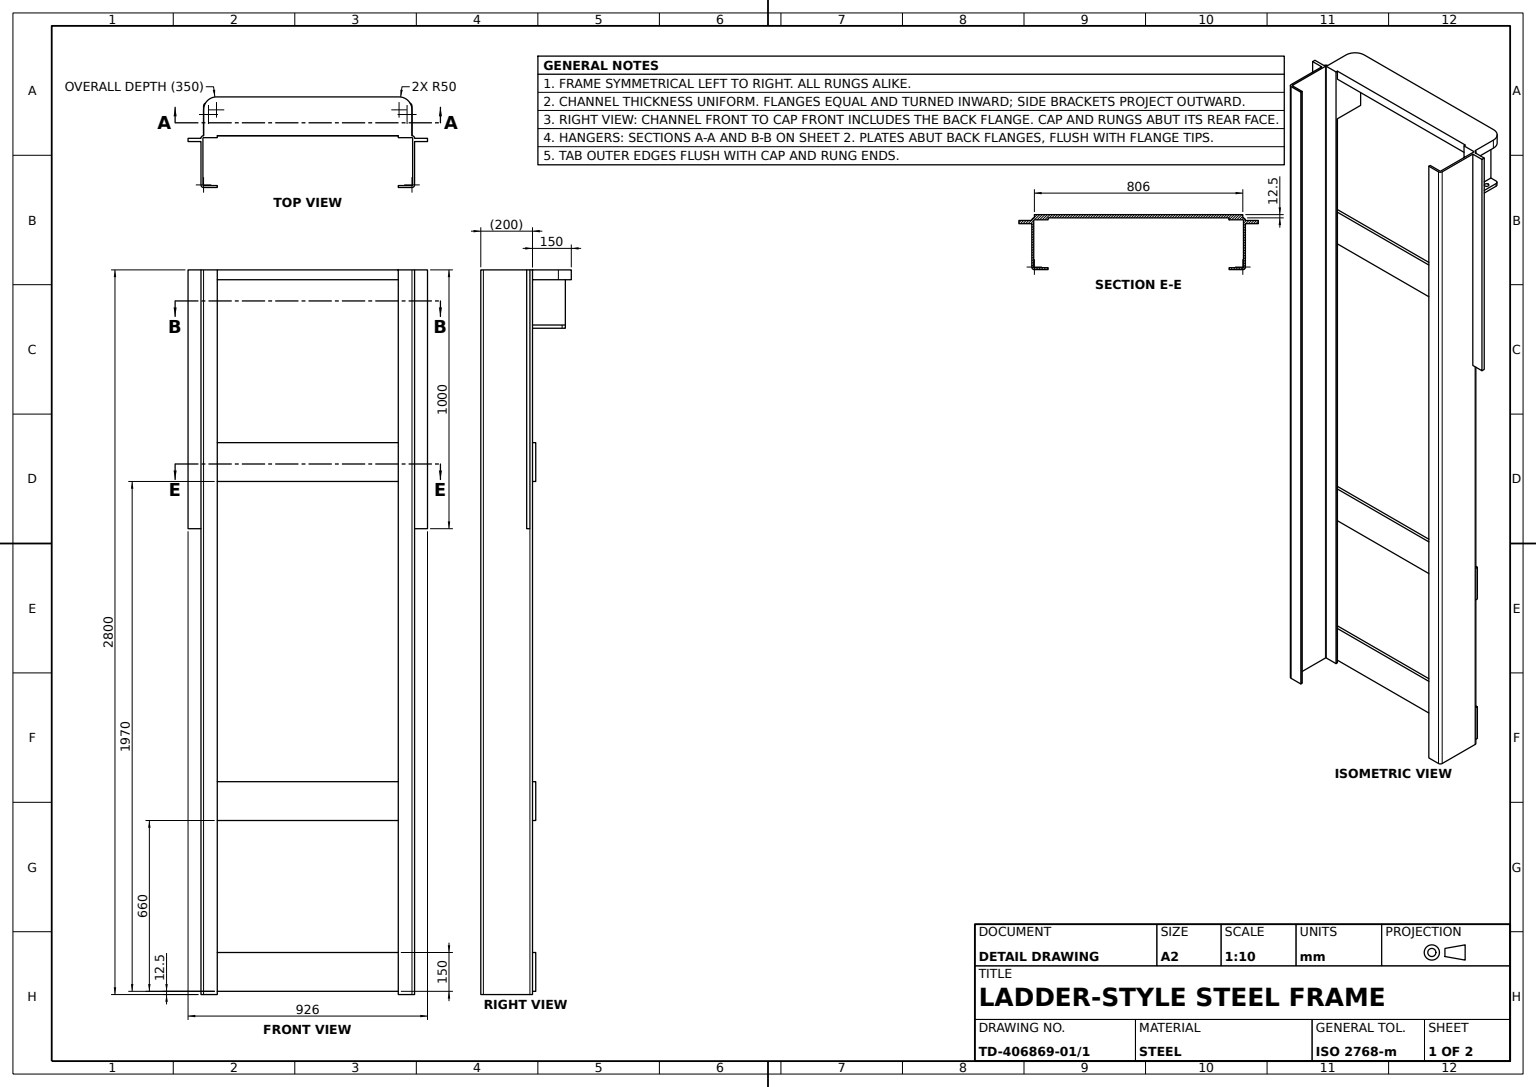
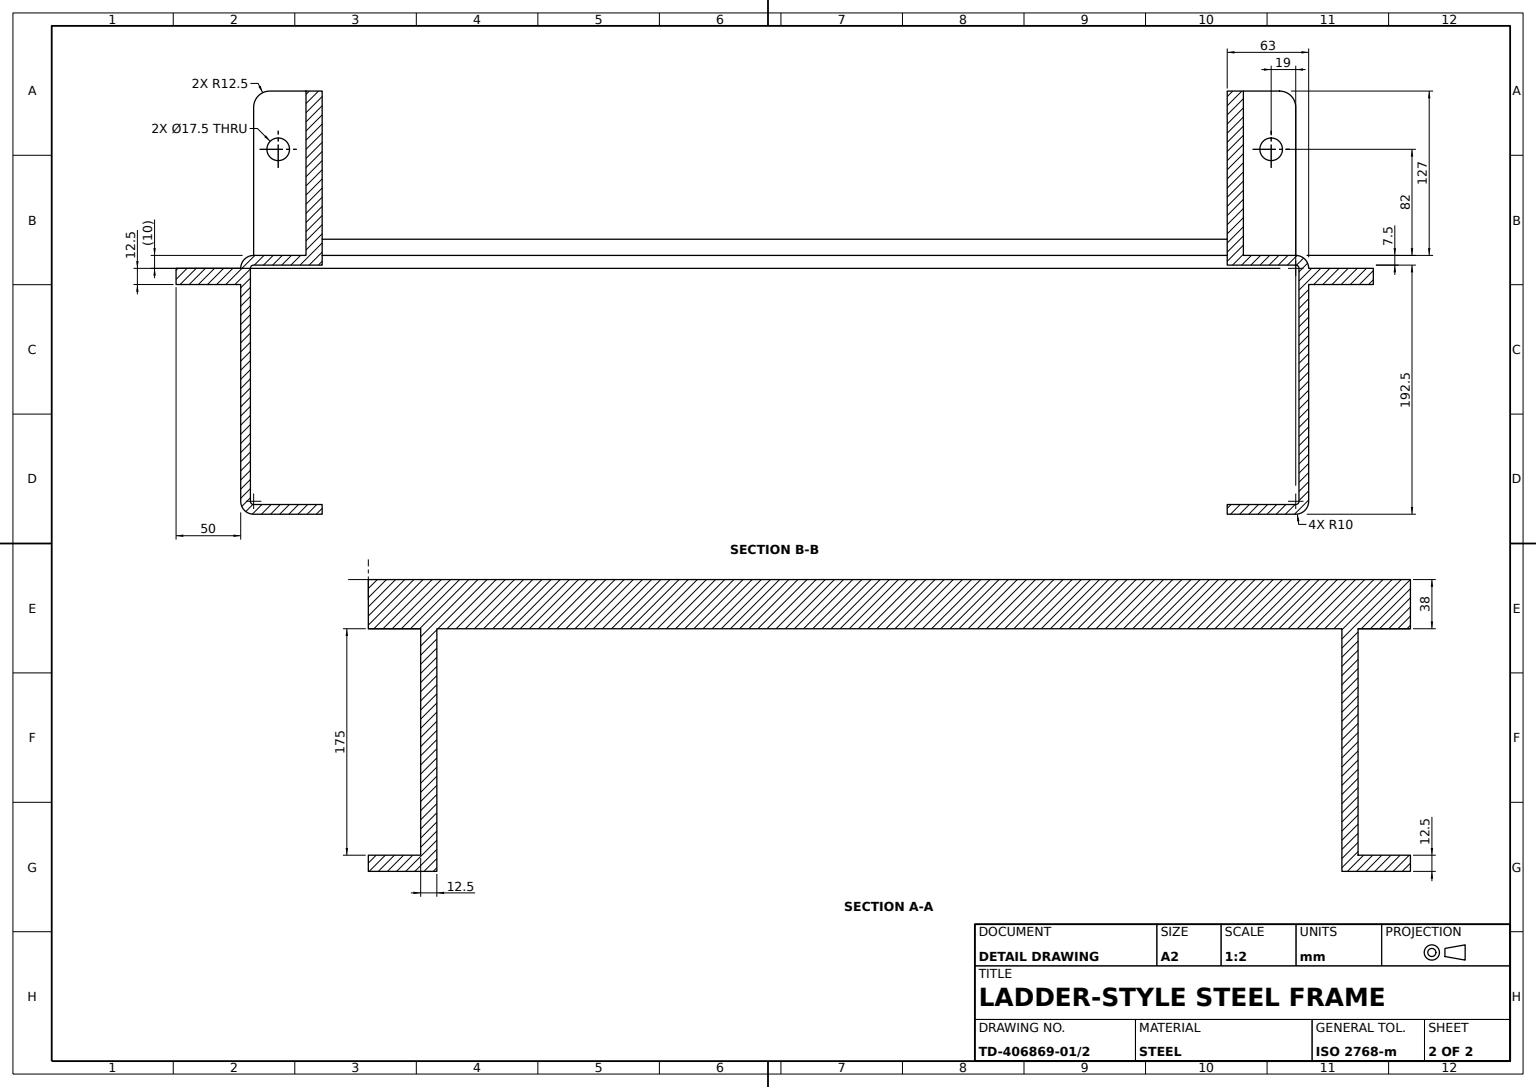
from build123d import *

# Parameters (mm, degrees)
SIDE_CHANNEL_RAIL_L2800_DEPTH = 1400
TOP_CAP_SKETCH_W              = 50
TOP_CAP_SKETCH_H              = 12.5
TOP_CAP_PLATE_DEPTH           = 1000
SIDE_BRACKET_DEPTH            = 38
CROSS_BAR_SKETCH_W            = 806
CROSS_BAR_SKETCH_H            = 150
CROSS_BAR_DEPTH               = 12.5
CROSS_BAR_PATTERN_660_COUNT   = 2
CROSS_BAR_PATTERN_660_PITCH   = 660
CROSS_BAR_PATTERN_1970_COUNT  = 2
CROSS_BAR_PATTERN_1970_PITCH  = 1970
HANGER_PLATE_SKETCH_W         = 12.5
HANGER_PLATE_SKETCH_H         = 127
HANGER_PLATE_DEPTH            = 175
HANGER_TAB_SKETCH_W           = 53
HANGER_TAB_SKETCH_H           = 127
HANGER_TAB_SKETCH_R           = 8.75
HANGER_TAB_DEPTH              = 12.5
HANGER_TAB_FILLET_R12_5_R     = 12.5


with BuildPart() as part:
    # Side Channel Profile Sketch → Side Channel Rail L2800 (new, symmetric)
    with BuildSketch(Plane(origin=(0, 0, 0), x_dir=(1, 0, 0), z_dir=(0, 1, 0))):
        with BuildLine():
            Line((350, 100), (403, 100))
            ThreePointArc((403, 100), (410.071067812, 97.071067812), (413, 90))
            Line((413, 90), (413, -90))
            ThreePointArc((413, -90), (410.071067812, -97.071067812), (403, -100))
            Line((403, -100), (350, -100))
            Line((350, -100), (350, -92.5))
            Line((350, -92.5), (403, -92.5))
            ThreePointArc((403, -92.5), (404.767766953, -91.767766953), (405.5, -90))
            Line((405.5, -90), (405.5, 90))
            ThreePointArc((405.5, 90), (404.767766953, 91.767766953), (403, 92.5))
            Line((403, 92.5), (350, 92.5))
            Line((350, 92.5), (350, 100))
        make_face()
    extrude(amount=SIDE_CHANNEL_RAIL_L2800_DEPTH, both=True)

    # Top Cap Sketch → Top Cap Plate (add)
    with BuildSketch(Plane(origin=(0, 1400, 0), x_dir=(1, 0, 0), z_dir=(0, 1, 0))):
        with Locations((438, 83.75)):
            Rectangle(TOP_CAP_SKETCH_W, TOP_CAP_SKETCH_H)
    extrude(amount=-TOP_CAP_PLATE_DEPTH)


with BuildPart() as body_2:
    # Side Rail Mirror: mirrored copy
    add(part.part.mirror(Plane(origin=(0, 0, 0), x_dir=(0, 0, 1), z_dir=(1, 0, 0))))


with BuildPart() as part_1:
    add(part.part)

    add(body_2.part)  # Side Bracket merges body 2
    # Bracket Sketch → Side Bracket (add)
    with BuildSketch(Plane(origin=(0, 1400, 0), x_dir=(1, 0, 0), z_dir=(0, 1, 0))):
        with BuildLine():
            Line((-403, 100), (403, 100))
            Line((403, 100), (403, 200))
            ThreePointArc((403, 200), (388.355339059, 235.355339059), (353, 250))
            Line((353, 250), (-353, 250))
            ThreePointArc((-353, 250), (-388.355339059, 235.355339059), (-403, 200))
            Line((-403, 200), (-403, 100))
        make_face()
    extrude(amount=-SIDE_BRACKET_DEPTH)

    # Cross Bar Sketch → Cross Bar (add)
    with BuildSketch(Plane(origin=(0, 0, -100), x_dir=(-1, 0, 0), z_dir=(0, 0, -1))):
        with Locations((0, -1312.5)):
            Rectangle(CROSS_BAR_SKETCH_W, CROSS_BAR_SKETCH_H)
    cross_bar = extrude(amount=CROSS_BAR_DEPTH)

    # Cross Bar Pattern 660: Cross Bar ×2
    with Locations(*[(0, i * CROSS_BAR_PATTERN_660_PITCH, 0) for i in range(1, CROSS_BAR_PATTERN_660_COUNT)]):
        add(cross_bar)

    # Cross Bar Pattern 1970: Cross Bar ×2
    with Locations(*[(0, i * CROSS_BAR_PATTERN_1970_PITCH, 0) for i in range(1, CROSS_BAR_PATTERN_1970_COUNT)]):
        add(cross_bar)

    # Hanger Plate Sketch → Hanger Plate (add)
    with BuildSketch(Plane.XZ.offset(-1362)):
        with Locations((-356.25, -163.5)):
            Rectangle(HANGER_PLATE_SKETCH_W, HANGER_PLATE_SKETCH_H)
    extrude(amount=HANGER_PLATE_DEPTH)

    # Hanger Tab Sketch → Hanger Tab (add)
    with BuildSketch(Plane.XZ.offset(-1187)):
        with Locations((-376.5, -163.5)):
            Rectangle(HANGER_TAB_SKETCH_W, HANGER_TAB_SKETCH_H)
        with Locations(Location((-384, -182, 0), (0, 0, 270))):
            Circle(HANGER_TAB_SKETCH_R, mode=Mode.SUBTRACT)
    extrude(amount=HANGER_TAB_DEPTH)

    # Hanger Tab Fillet R12.5
    hanger_tab_fillet_r12_5_edges = [part_1.edges().sort_by_distance(p)[0] for p in [
        (-403, 1180.75, -227),
    ]]
    fillet(hanger_tab_fillet_r12_5_edges, radius=HANGER_TAB_FILLET_R12_5_R)

    # Side Bracket Mirror: part across plane


with BuildPart() as part_2:
    add(part_1.part)
    add(part_1.part.mirror(Plane(origin=(0, 0, 0), x_dir=(0, 0, 1), z_dir=(1, 0, 0))))


solid = part_2.part
